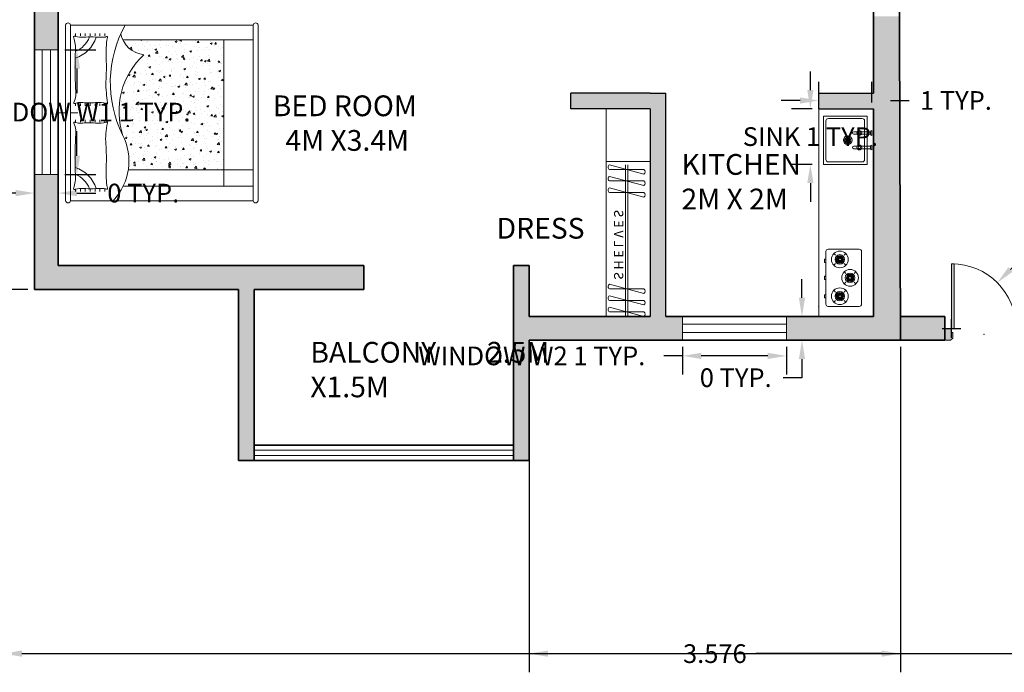
# Model space of a CAD drawing. Units: metres. Extents: x 2031 to 2061.8, y 1886.4 to 1909.8.
# Tile 2 of 10: x 2036.4 to 2045.9, y 1886.4 to 1892.7. Entities that reach past the tile are written whole.
import ezdxf

# ---------------------------------------------------------------- set-up
doc = ezdxf.new("R2010")
doc.units = ezdxf.units.M
for name, color, linetype, lineweight in [('A-ANNO-DIMS', 2, 'Continuous', 18), ('A-AREA-IDEN', 7, 'Continuous', 18), ('A-EQPM', 8, 'Continuous', 18), ('A-FLOR-CASE', 8, 'Continuous', 18), ('A-FLOR-FIXT', 8, 'Continuous', 18), ('A-WALL-PATT', 252, 'Continuous', 13), ('doors & windows', 30, 'Continuous', 18), ('furniture', 24, 'Continuous', 13), ('grills', 5, 'Continuous', 13), ('inner walls', 4, 'Continuous', 25), ('windows', 30, 'Continuous', 18)]:
    doc.layers.add(name, color=color, linetype=linetype, lineweight=lineweight)
doc.layers.add('outer walls', color=1, linetype='Continuous', lineweight=35, plot=False)
doc.styles.get("Standard").update_dxf_attribs({"font": 'arial.ttf'})
doc.dimstyles.get("Standard").update_dxf_attribs({"dimtxt": 0.18, "dimasz": 0.18, "dimexe": 0.18, "dimexo": 0.0625, "dimgap": 0.09, "dimtad": 0, "dimtih": 1, "dimtoh": 1, "dimdec": 4, "dimzin": 0, "dimdsep": 46, "dimtxsty": 'Standard', "dimcen": 0.09, "dimadec": 0, "dimazin": 0, "dimtfac": 1, "dimtdec": 4, "dimtofl": 0, "dimtmove": 0, "dimatfit": 3, "dimfxl": 1, "dimtolj": 1, "dimtzin": 0, "dimarcsym": 0})

# ---------------------------------------------------------------- blocks, each defined once
blk = doc.blocks.new('sink')
for p, q in [((0, 0), (-22.00000000000001, 0)), ((0, 0), (0, 0)), ((-20.00000000000023, -2.999999999999995), (-2.000000000000178, -3)), ((-19.99999999999959, -22.99999999999988), (-20.00000000000023, -2.999999999999995)), ((-18.00000000000017, -3.999999999999996), (-4.000000000000113, -3.999999999999999)), ((-2.000000000000178, -3), (-1.999999999999543, -22.99999999999988)), ((-18.99999999999966, -20.99999999999994), (-19.00000000000017, -4.999999999999996)), ((-3.000000000000114, -5), (-2.999999999999607, -20.99999999999988)), ((-0.5000000000000026, -9.499999999999813), (-7.500000000000004, -9.499999999999812)), ((-0.5000000000000028, -10.49999999999981), (-7.500000000000004, -10.49999999999981)), ((-0.5000000000000026, -9.499999999999813), (-0.5000000000000028, -10.49999999999981)), ((-2.4e-15, -8.999999999999813), (-2.9e-15, -10.99999999999981)), ((-0.500000000000004, -15.49999999999981), (-7.500000000000005, -15.49999999999981)), ((-0.500000000000004, -15.49999999999981), (-0.5000000000000044, -16.49999999999981)), ((-3.9e-15, -14.99999999999981), (-4.4e-15, -16.99999999999981)), ((-0.5000000000000044, -16.49999999999981), (-7.500000000000005, -16.49999999999981)), ((-19.99999999999959, -22.99999999999988), (-1.999999999999543, -22.99999999999988)), ((-17.99999999999966, -21.99999999999988), (-3.999999999999607, -21.99999999999989))]:
    blk.add_line(p, q)
for centre, radius in [((-10.00000000000014, -12.99999999999968), 1.794435724606955), ((-10.00000000000014, -12.99999999999968), 1.294435724606955), ((-10.00000000000014, -12.23682250650668), 0.25), ((-5.180961460384426, -9.999999999999812), 1), ((-5.180961460384426, -9.999999999999812), 0.5), ((-10.66093109696162, -12.61841125325318), 0.25), ((-10.66093109696162, -13.38158874674618), 0.25), ((-10.00000000000014, -12.99999999999968), 0.25), ((-10.00000000000014, -13.76317749349269), 0.25), ((-9.33906890303867, -12.61841125325318), 0.25), ((-9.33906890303867, -13.38158874674618), 0.25), ((-5.180961460384427, -15.99999999999981), 1), ((-5.180961460384427, -15.99999999999981), 0.5)]:
    blk.add_circle(centre, radius)
for centre, radius, start, end in [((-18.00000000000017, -4.999999999999996), 1, 89.99999999999999, 180), ((-4.000000000000115, -5), 1, 0, 89.99999999999999), ((-7.500000000000004, -9.999999999999812), 0.5, 89.99999999999999, 270), ((0.010449978117122, -9.510449978116938), 0.5105569333604445, 91.17280055555744, 178.8271994444424), ((0.0104499781171218, -10.48955002188269), 0.5105569333604445, 181.1728005555574, 268.8271994444423), ((-7.500000000000005, -15.99999999999981), 0.5, 89.99999999999999, 270), ((0.0104499781171206, -15.51044997811693), 0.5105569333604445, 91.17280055555744, 178.8271994444424), ((0.0104499781171203, -16.48955002188269), 0.5105569333604445, 181.1728005555573, 268.8271994444423), ((-17.99999999999966, -20.99999999999988), 1, 180, 270), ((-3.999999999999607, -20.99999999999988), 1, 270, 0)]:
    blk.add_arc(centre, radius, start, end)
blk = doc.blocks.new('stove')
at = {"layer": 'furniture'}
h = blk.add_hatch(dxfattribs=at)
h.set_pattern_fill('HEX', color=256, angle=180, style=0)
h.set_pattern_definition([(360, (23.99999999999982, 24.99999999999816), (1e-16, 0.216506351), [0.125, -0.25]), (119.9999999999999, (23.99999999999982, 24.99999999999816), (-0.1875000000466704, -0.1082531754999999), [0.1249999999999998, -0.2499999999999996]), (59.99999999999994, (24.12499999999982, 24.99999999999816), (-0.1875000000466704, 0.1082531755000001), [0.125, -0.25])])
h.paths.add_polyline_path([(10.36428182591571, 19.71316705046143, 1), (7.364281825915714, 19.71316705046143, 1)])
h.paths.add_polyline_path([(9.364281825915715, 19.71316705046143, -1), (8.364281825915715, 19.71316705046143, -1)], flags=16)
h = blk.add_hatch(dxfattribs=at)
h.set_pattern_fill('HEX', color=256, angle=180, style=0)
h.set_pattern_definition([(180, (-2.000000000000001, 6.713167050462818), (-1e-16, -0.216506351), [0.125, -0.25]), (300, (-2.000000000000001, 6.713167050462818), (0.1875000000466704, 0.1082531754999999), [0.1249999999999999, -0.2499999999999998]), (239.9999999999999, (-2.125000000000001, 6.713167050462818), (0.1875000000466704, -0.1082531755000001), [0.125, -0.25])])
h.paths.add_polyline_path([(14.6357181740841, 11.99999999999954, 1), (11.6357181740841, 11.99999999999954, 1)])
h.paths.add_polyline_path([(12.6357181740841, 11.99999999999954, -1), (13.6357181740841, 11.99999999999954, -1)], flags=16)
h = blk.add_hatch(dxfattribs=at)
h.set_pattern_fill('HEX', color=256, angle=180, style=0)
h.set_pattern_definition([(360, (23.99999999999982, -0.9999999999999342), (-1e-16, -0.216506351), [0.125, -0.25]), (239.9999999999999, (23.99999999999982, -0.9999999999999342), (-0.1875000000466704, 0.1082531755), [0.1249999999999999, -0.2499999999999998]), (300, (24.12499999999982, -0.9999999999999342), (-0.1875000000466704, -0.1082531755), [0.125, -0.2499999999999999])])
h.paths.add_polyline_path([(10.36428182591571, 4.2868329495368, 1), (7.364281825915714, 4.2868329495368, 1)])
h.paths.add_polyline_path([(9.364281825915715, 4.2868329495368, -1), (8.364281825915715, 4.2868329495368, -1)], flags=16)
for p, q in [((3, 1.000000000000003), (3.000000000000007, 22.99999999999909)), ((4.000000000000007, 23.99999999999909), (17, 23.99999999999908)), ((6.389408091762671, 22.18804078461422), (7.09651487294905, 21.48093400342751)), ((10.6320487788818, 21.48093400342809), (11.33915556006851, 22.18804078461447)), ((18, 22.99999999999908), (18, 0.9999999999991327)), ((3.000000000000007, 19.86017834974973), (2.500000000000003, 19.86017834974973)), ((2.500000000000003, 19.86017834974973), (2.500000000000003, 18.36017834974973)), ((2.500000000000003, 18.36017834974973), (3.000000000000003, 18.36017834974973)), ((6.389408091762675, 17.23829331630864), (7.096514872949061, 17.94540009749535)), ((10.63204877888179, 17.94540009749477), (11.3391555600685, 17.23829331630838)), ((2.500000000000003, 12.64999999999954), (2.500000000000003, 11.34999999999955)), ((3.000000000000003, 12.64999999999954), (2.500000000000003, 12.64999999999954)), ((11.36795122111803, 13.7677669529662), (10.66084443993131, 14.47487373415259)), ((15.61059190823715, 14.47487373415233), (14.90348512705075, 13.76776695296562)), ((2.500000000000003, 11.34999999999955), (3.000000000000003, 11.34999999999955)), ((11.36795122111803, 10.23223304703288), (10.66084443993131, 9.525126265846504)), ((15.61059190823714, 9.525126265846753), (14.90348512705077, 10.23223304703346)), ((2.500000000000003, 4.936832949536799), (2.500000000000003, 3.636832949536802)), ((3.000000000000003, 4.936832949536799), (2.500000000000003, 4.936832949536799)), ((6.389408091762671, 6.761706683689592), (7.096514872949061, 6.054599902502877)), ((10.63204877888178, 6.05459990250346), (11.3391555600685, 6.761706683689842)), ((2.500000000000003, 3.636832949536802), (3.000000000000003, 3.636832949536802)), ((16.99999999999994, -8.669e-13), (3.999999999999946, 3.6e-15)), ((6.389408091762668, 1.811959215384014), (7.096514872949043, 2.519065996570723)), ((10.63204877888179, 2.519065996570138), (11.3391555600685, 1.81195921538376))]:
    blk.add_line(p, q, dxfattribs=at)
for centre, radius in [((8.864281825915715, 19.71316705046143), 3.499999999999999), ((8.864281825915715, 19.71316705046143), 1.999999999999999), ((8.864281825915715, 19.71316705046143), 1.5), ((8.864281825915715, 19.71316705046143), 0.5000000000000004), ((13.1357181740841, 11.99999999999954), 3.499999999999999), ((13.1357181740841, 11.99999999999954), 1.999999999999999), ((13.1357181740841, 11.99999999999954), 1.5), ((13.1357181740841, 11.99999999999954), 0.5000000000000004), ((8.864281825915715, 4.286832949536801), 3.499999999999999), ((8.864281825915715, 4.2868329495368), 1.999999999999999), ((8.864281825915715, 4.2868329495368), 1.5), ((8.864281825915715, 4.2868329495368), 0.5000000000000004)]:
    blk.add_circle(centre, radius, dxfattribs=at)
for centre, start, end in [((4.000000000000007, 22.99999999999909), 90, 180), ((17, 22.99999999999908), 0, 90), ((4, 1.000000000000003), 180, 269.9999999999968), ((17, 0.9999999999991331), 269.9999999999968, 0)]:
    blk.add_arc(centre, 1, start, end, dxfattribs=at)
at = {"layer": 'furniture', "ltscale": 9}
blk.add_point((0, 0), dxfattribs=at)
blk = doc.blocks.new('bed')
at = {"layer": 'furniture'}
h = blk.add_hatch(dxfattribs=at)
h.set_pattern_fill('AR-CONC', color=256, angle=-90.00000000000003, style=0)
h.set_pattern_definition([(320, (0, 2.380000000001032), (-0.6275213498259539, -7.172601826007534), [0.75, -8.25]), (265, (0, 2.380000000001032), (7.521921337000119, 1.387513336129997), [0.6, -6.599999999999999]), (10.45139999999999, (-0.0522933999999964, 1.782283200001032), (6.894395420609534, -5.785093817140218), [0.6374019000000001, -7.011421119999999]), (316.1842, (2, 2.380000000001032), (-1.655190143290184, -10.67241048625644), [1.125, -12.375]), (6.635599999999979, (1.862066929999997, 1.490632550001038), (9.741178709004412, -9.346627055487035), [0.956102879999999, -10.51712999999998]), (261.1842, (2, 2.380000000001032), (9.741186009253243, -9.346619451336275), [0.8999999999999989, -9.899999999999984]), (291, (1.5, 1.380000000001032), (-4.02618890665339, -5.969070521184614), [0.75, -8.25]), (236, (1.5, 1.380000000001032), (7.251500450468529, -2.433153319215819), [0.6, -6.599999999999999]), (341.4514, (1.164483939999996, 0.8825776700010266), (3.22530496709952, -8.402226285814901), [0.6374019000000001, -7.011421119999999]), (307.4999999999999, (0, 2.380000000001032), (3.328938538313114, -0.121598553172908), [0, -6.519999999999999, 0, -6.7, 0, -6.625]), (277.5, (0, 2.380000000001032), (3.944117118823601, -2.630695374421487), [0, -3.819999999999999, 0, -6.37, 0, -2.524999999999999]), (237.5, (0, 4.610000000001036), (-0.2255487173438, -5.33822436172409), [0, -2.5, 0, -7.799999999999999, 0, -10.35]), (227.5, (0, 5.610000000001036), (1.001049823323174, -5.831861693423862), [0, -3.25, 0, -5.179999999999999, 0, -7.349999999999999])])
h.paths.add_polyline_path([(30.01221964123038, -67.99999999999999), (30.01221964123036, -26.4972098666525, 0.2630430180581192), (23.90476957024844, -35.1500155485824, 0.2934236934375176), (-9.177957282599145, -26.46678060096597, -0.1566832162072435), (-23.39221964123496, -28.71851562074189), (-23.39221964123494, -67.99999999999999)])
for p, q in [((0, -3), (0, 0)), ((36.01221964123033, -3), (-36.01221964123033, -3)), ((-36.01221964123033, -5.000000000000028), (-36.01221964123027, -80)), ((36.01221964123033, -5.000000000000042), (-36.01221964123033, -5.000000000000028)), ((-31.23716250644156, -7.067621994530554), (-32.23716250644157, -7.067621994530554)), ((-3.810600647213163, -7.067621994530554), (-2.810600647213163, -7.067621994530554)), ((0, -8.000000000000043), (0, -5.000000000000042)), ((3.894900133777696, -7.067621994530526), (2.894900133777696, -7.067621994530526)), ((31.62837541028949, -7.067621994530526), (32.62837541028949, -7.067621994530526)), ((36.01221964123039, -79.99999999999999), (36.01221964123033, -5.000000000000042)), ((-31.23716250644156, -9.067621994530555), (-32.23716250644157, -9.067621994530555)), ((-31.23716250644156, -11.06762199453055), (-32.23716250644157, -11.06762199453055)), ((-3.810600647213163, -9.067621994530555), (-2.810600647213163, -9.067621994530555)), ((-3.810600647213163, -11.06762199453055), (-2.810600647213163, -11.06762199453055)), ((3.894900133777696, -9.067621994530526), (2.894900133777696, -9.067621994530526)), ((3.894900133777696, -11.06762199453052), (2.894900133777696, -11.06762199453052)), ((31.62837541028949, -9.067621994530526), (32.62837541028949, -9.067621994530526)), ((31.62837541028949, -11.06762199453052), (32.62837541028949, -11.06762199453052)), ((-31.23716250644156, -13.06762199453055), (-32.23716250644157, -13.06762199453055)), ((-31.23716250644156, -15.06762199453055), (-32.23716250644157, -15.06762199453055)), ((-3.810600647213163, -13.06762199453055), (-2.810600647213163, -13.06762199453055)), ((-3.810600647213163, -15.06762199453055), (-2.810600647213163, -15.06762199453055)), ((3.894900133777696, -13.06762199453052), (2.894900133777696, -13.06762199453052)), ((3.894900133777696, -15.06762199453052), (2.894900133777696, -15.06762199453052)), ((31.62837541028949, -13.06762199453052), (32.62837541028949, -13.06762199453052)), ((31.62837541028949, -15.06762199453052), (32.62837541028949, -15.06762199453052)), ((-31.23716250644156, -17.06762199453055), (-32.23716250644157, -17.06762199453055)), ((-31.23716250644156, -19.06762199453055), (-32.23716250644157, -19.06762199453055)), ((-3.810600647213163, -17.06762199453055), (-2.810600647213163, -17.06762199453055)), ((-3.810600647213163, -19.06762199453055), (-2.810600647213163, -19.06762199453055)), ((3.894900133777696, -17.06762199453052), (2.894900133777696, -17.06762199453052)), ((3.894900133777696, -19.06762199453052), (2.894900133777696, -19.06762199453052)), ((31.62837541028949, -17.06762199453052), (32.62837541028949, -17.06762199453052)), ((31.62837541028949, -19.06762199453052), (32.62837541028949, -19.06762199453052)), ((-36.01221964123027, -80), (36.01221964123039, -79.99999999999997)), ((-36.01221964123027, -82), (36.01221964123039, -82))]:
    blk.add_line(p, q, dxfattribs=at)
at = {"layer": 'furniture', "ltscale": 5}
blk.add_line((-30.0122196412303, -26.65900214866815), (-30.01221964123028, -80), dxfattribs=at)
at = {"layer": 'furniture', "ltscale": 7}
blk.add_line((30.01221964123039, -79.99999999999999), (30.01221964123036, -26.4972098666525), dxfattribs=at)
at = {"layer": 'furniture', "ltscale": 0.3}
for p, q in [((-23.39221964123493, -80.00000000000003), (-23.39221964123496, -28.71851562074188)), ((-30.01221964123028, -67.99999999999999), (30.01221964123039, -67.99999999999999))]:
    blk.add_line(p, q, dxfattribs=at)
at = {"layer": 'furniture'}
for centre, radius, start, end in [((-35.95310404783035, -4.000000000000014), 1.001745802777857, 93.38313670775338, 266.6168632922466), ((35.95310404783047, -4.000000000000014), 1.001745802777857, 273.3831367077534, 86.61686329224663), ((-31.09685452420217, -6.56812628935117), 0.3815901177143176, 35.89755946985184, 208.6271807330242), ((-44.4434251214767, -13.85312857714783), 14.82374463825802, 27.16285943351717, 28.62718073212637), ((-46.75951437957865, -9.65138206848897), 15.71579241958107, 357.4803608088326, 9.395608387614068), ((-34.45294545533051, -3.506108501804959), 9.853247350176973, 289.8695209624031, 338.9842964810487), ((-34.45294545533051, -3.506108501804959), 12.47479548168961, 286.0319050224358, 344.1205283884622), ((-26.34909713879518, 6.677823774407073), 13.75788850886336, 251.1782289026713, 273.3982224065857), ((-18.01528168092849, -163.5963416214672), 156.7209082093599, 87.00321809951629, 92.74968346925495), ((-8.031939823939297, 2.030581047412752), 9.294330538692307, 258.8960367609226, 294.7184225587751), ((0.254091396095987, -8.800915214962217), 4.494229367051207, 159.014640107615, 186.2730421081171), ((-4.029449448298862, -6.668977911985379), 0.2818061021667602, 335.7259061638442, 114.3030308467571), ((3.223958981487498, -9.94006998173215), 7.675076275868892, 155.7259061638442, 159.0146401085631), ((4.113748934860268, -6.668977911985379), 0.2818061021635516, 65.69696915417202, 204.2740938370052), ((-3.139659494904833, -9.940069981732137), 7.675076275868892, 20.98535989143595, 24.27409383615427), ((-0.1697919095242355, -8.800915214962217), 4.494229367051207, 353.7269578918828, 20.98535989238499), ((8.116239310533615, 2.030581047735168), 9.294330539002221, 245.2815774418415, 281.1039632384965), ((18.09958116748922, -163.5963416214399), 156.7209082093326, 87.2503165307418, 92.99678190048373), ((34.53724494190226, -3.506108501789682), 12.47479548168961, 195.8794716115377, 253.9680949775642), ((34.53724494190226, -3.506108501789682), 9.853247350176973, 201.0157035189505, 250.1304790375968), ((26.43339662535652, 6.677823774423444), 13.75788850886336, 266.6017775934111, 288.8217710973251), ((31.18115401076358, -6.568126289351184), 0.3815901177179044, 331.3728192669758, 144.1024405301472), ((46.84381386614001, -9.651382068520647), 15.71579241958353, 170.6043916115409, 182.5196391911672), ((44.52772460803806, -13.85312857714784), 14.82374463825802, 151.3728192678729, 152.8371405664821), ((-28.61556435462791, 31.03444768063454), 42.31456350822244, 266.4835611990511, 266.6487421238194), ((54.88285648445511, -13.16191061182081), 85.98801403775587, 178.1208768196816, 183.3613129440673), ((-32.81622258778788, -12.43616332427339), 28.77528664700029, 354.3784002715227, 6.27304210895588), ((32.90052207435963, -12.43616332427341), 28.77528664700055, 173.7269578910441, 185.6215997284773), ((-54.79855699787332, -13.1619106118885), 85.98801403775471, 356.6386870559327, 1.87912318031836), ((28.69986384117891, 31.03444768073385), 42.31456350831875, 273.3512578762066, 273.5164388009489), ((12.27920019974715, -16.10835590841725), 16.48064095036883, 177.0317121189266, 192.8677860199701), ((-12.19490071317551, -16.10835590841725), 16.48064095036894, 347.1322139800299, 2.968287881073314), ((-31.05019458355673, -19.91479358257859), 0.2912925215689113, 147.6219291273817, 311.93432899363), ((-33.19532486499685, -18.55460390606353), 2.248727139855352, 327.6219291288709, 339.224552802207), ((-34.12771521855714, -18.41167218428833), 3.177308659740759, 342.7808628527732, 3.755021134780372), ((-24.39731400277299, -58.0065508966982), 38.42172354635978, 93.51643880178425, 99.67664784205135), ((-24.51665474671893, -56.06449133928439), 36.47600066328987, 86.48356119821578, 93.51643880178425), ((-18.48842024981553, 70.49496359167773), 90.23180174042126, 267.5920770069633, 273.6328801943956), ((-10.30534078399284, -44.95285539311296), 25.51674577343078, 75.95197577712642, 95.54518109318596), ((-3.947726608991956, -19.99033763805275), 0.2654728058058112, 231.9004795059564, 52.89022406852256), ((4.032026095563765, -19.99033763805275), 0.2654728058058112, 127.1097759314774, 308.0995204940429), ((7.570216687580227, -34.67789736270967), 14.86666553287629, 87.39755039330738, 103.1191401867811), ((11.43897390287765, -34.80624327566366), 15.31635237680183, 84.69404282866213, 102.035481886755), ((18.57271973638731, 70.4949635916777), 90.23180174042125, 266.3671198056044, 272.4079229930367), ((24.6009542333012, -56.0644913392844), 36.47600066328987, 86.48356119821578, 93.51643880178425), ((24.48161348934542, -58.00655089669821), 38.42172354635978, 80.32335215794863, 86.48356119821578), ((31.13449407013883, -19.91479358255678), 0.2912925215689113, 228.06567100637, 32.37807087261824), ((34.21201470513921, -18.41167218428845), 3.177308659740705, 176.2449788652196, 197.2191371472267), ((33.27962435157895, -18.55460390604825), 2.248727139855352, 200.775447197793, 212.378070871129), ((-19.78970084288576, -5.469494448941333), 23.52647715105876, 226.4060518471351, 297.4441169484015), ((12.50744191168894, -69.71437404891591), 48.3828132966499, 60.93454900685955, 116.3226601669859), ((0.602167516954296, -56.56840710701565), 31.65057281321388, 42.58740832788977, 108.5033645785765), ((34.6132349005153, -36.22659364526982), 10.76244628919441, 101.1719081394, 174.2590453022261), ((-35.95310404783035, -81), 1.001745802777857, 93.38313670775338, 266.6168632922466), ((35.95310404783044, -81), 1.001745802777857, 273.3831367077534, 86.61686329224663)]:
    blk.add_arc(centre, radius, start, end, dxfattribs=at)
blk = doc.blocks.new('hangers')
at = {"layer": 'furniture'}
for p, q in [((1.8e-15, 16.5), (4.000000000000001, 1.5)), ((2.000000000000001, 16.5), (2.000000000000001, 1.5)), ((5.000000000000001, 16.5), (9.000000000000002, 1.5)), ((7.000000000000001, 16.5), (7.000000000000001, 1.5)), ((10, 16.5), (14, 1.5)), ((12, 16.5), (12, 1.5)), ((52, 16.5), (56, 1.5)), ((54, 16.5), (54, 1.5)), ((57, 16.5), (61, 1.5)), ((59, 16.5), (59, 1.5)), ((62, 16.5), (66, 1.5)), ((64, 16.5), (64, 1.5)), ((66, 9.5), (1.8e-15, 9.5)), ((1.8e-15, 8.5), (66, 8.5))]:
    blk.add_line(p, q, dxfattribs=at)
for centre, radius, start, end in [((1.000000000000001, 15.6218374153911), 1.33085293139661, 41.28839256573093, 138.711607434269), ((6.000000000000001, 15.6218374153911), 1.33085293139661, 41.28839256573093, 138.711607434269), ((11, 15.6218374153911), 1.33085293139661, 41.28839256573093, 138.711607434269), ((53, 15.6218374153911), 1.33085293139661, 41.28839256573107, 138.7116074342689), ((58, 15.6218374153911), 1.33085293139661, 41.28839256573107, 138.7116074342689), ((63, 15.6218374153911), 1.33085293139661, 41.28839256573107, 138.7116074342689), ((3.000000000000001, 1.915335972440686), 1.082822224561017, 202.5548696812492, 337.4451303187508), ((8.000000000000002, 1.915335972440686), 1.082822224561017, 202.5548696812492, 337.4451303187508), ((13, 1.915335972440686), 1.082822224561017, 202.5548696812492, 337.4451303187508), ((55, 1.915335972440686), 1.082822224561017, 202.5548696812491, 337.4451303187509), ((60, 1.915335972440686), 1.082822224561017, 202.5548696812491, 337.4451303187509), ((65, 1.915335972440686), 1.082822224561017, 202.5548696812491, 337.4451303187509)]:
    blk.add_arc(centre, radius, start, end, dxfattribs=at)
blk.add_point((0, 0), dxfattribs=at)
blk.add_text('S H E L V E S', height=4, dxfattribs=at).set_placement((15.9969173169515, 3.475366291579639))
blk = doc.blocks.new('D2')
at = {"layer": 'doors & windows'}
h = blk.add_hatch(dxfattribs=at)
h.set_pattern_fill('DOTS', color=256, scale=2, angle=180, style=0)
h.set_pattern_definition([(180, (0, -3.999999999998181), (-0.0625, -0.125), [0, -0.125])])
h.paths.add_polyline_path([(2.5, 1.819e-12), (3.5, 1.819e-12), (3.500000000001818, 24.97999199359535, 0.0100030022021123), (2.500000000001818, 25.00000000000182)])
h = blk.add_hatch(dxfattribs=at)
h.set_pattern_fill('DOTS', color=256, scale=2, angle=180, style=0)
h.set_pattern_definition([(180, (0, 0), (-0.0625, -0.125), [0, -0.125])])
edge = h.paths.add_edge_path()
edge.add_line((27.50000000000182, 1.819e-12), (27.50000000000182, -1.499999999998181))
edge.add_line((27.50000000000182, -1.499999999998181), (27.00000000000157, -1.499999999998181))
edge.add_line((27.00000000000157, -1.499999999998181), (27.00000000000039, -3.749999999998181))
edge.add_line((27.00000000000039, -3.749999999998181), (27.25, -3.749999999998181))
edge.add_arc((27.75893604593965, -3.741063954058532), 0.5090144907305875, 181.0059124648427, 268.9940875351573)
edge.add_line((27.75, -4.249999999998181), (27.75, -4.499999999998181))
edge.add_line((27.75, -4.499999999998181), (30.00000000000182, -4.499999999998181))
edge.add_line((30.00000000000182, -4.499999999998181), (30.00000000000182, 0))
edge.add_line((30.00000000000182, 0), (27.50000000000182, 1.819e-12))
edge = h.paths.add_edge_path()
edge.add_line((2.5, -1.499999999998181), (2.5, 1.819e-12))
edge.add_line((2.5, 1.819e-12), (1.819e-12, 0))
edge.add_line((1.819e-12, 0), (0, -4.499999999998181))
edge.add_line((0, -4.499999999998181), (2.250000000001548, -4.499999999998181))
edge.add_line((2.250000000001548, -4.499999999998181), (2.250000000001548, -4.249999999998181))
edge.add_arc((2.2410639540619, -3.741063954058532), 0.5090144907305875, 271.0059124648427, 358.9940875351573)
edge.add_line((2.750000000001548, -3.749999999998181), (3, -3.749999999998181))
edge.add_line((3, -3.749999999998181), (3, -1.499999999998181))
edge.add_line((3, -1.499999999998181), (2.5, -1.499999999998181))
for p, q in [((1.819e-12, 0), (0, -4.499999999998181)), ((30.00000000000182, 0), (30.00000000000182, -4.499999999998181))]:
    blk.add_line(p, q)
blk.add_lwpolyline([(3.5, 1.819e-12), (3.500000000001818, 25.00000000000182), (2.500000000001818, 25.00000000000182), (2.5, 1.819e-12)], close=True, dxfattribs=at)
for points in [[(3, -3.749999999998181), (3, -1.499999999998181), (2.5, -1.499999999998181), (2.5, 1.819e-12), (1.819e-12, 0)], [(27.00000000000039, -3.749999999998181), (27.00000000000182, -1.499999999998181), (27.50000000000182, -1.499999999998181), (27.50000000000182, 1.819e-12), (30, 0)], [(0, -4.499999999998181), (2.250000000001548, -4.499999999998181)], [(30, -4.499999999998181), (27.75, -4.499999999998181)]]:
    blk.add_lwpolyline(points, dxfattribs=at)
for points in [[(2.250000000001548, -4.499999999998181), (2.250000000001548, -4.249999999998181, 0.4039662087126686), (2.750000000001548, -3.749999999998181), (3.000000000001548, -3.749999999998181)], [(27.75, -4.499999999998181), (27.75, -4.249999999998181, -0.4039662087126686), (27.25, -3.749999999998181), (27, -3.749999999998181)]]:
    blk.add_lwpolyline(points, format="xyb", dxfattribs=at)
at = {"layer": 'doors & windows', "ltscale": 6}
blk.add_arc((2.5, 1.819e-12), 25, 0, 90, dxfattribs=at)
at = {"layer": 'doors & windows'}
blk.add_point((15, -2.24999999999909), dxfattribs=at)
blk = doc.blocks.new('WIN-1200')
for p, q in [((0.2299999999995634, 1.200000000000045), (-4.547e-13, 1.199999999999818)), ((0.0750000000007276, -2.274e-13), (0.0749999999995907, 1.200000000000045)), ((0.1550000000006548, -2.274e-13), (0.154999999999518, 1.200000000000045)), ((0.2300000000007003, 0), (6.821e-13, -2.274e-13))]:
    blk.add_line(p, q)
blk = doc.blocks.new('WIN-1000')
for p, q in [((2.274e-13, 0), (0, 0.2299999999997908)), ((1.000000000000227, 9.095e-13), (1, 0.2300000000007003)), ((2.274e-13, 0.1549999999997453), (1.000000000000227, 0.1549999999997453)), ((2.274e-13, 0.0749999999998181), (1.000000000000227, 0.0749999999998181))]:
    blk.add_line(p, q)
blk = doc.blocks.new('BALCONY-GUARD-2500')
for p, q in [((4.547e-13, 0.0500000000010914), (2.5, 0.0500000000006367)), ((4.547e-13, 6.821e-13), (2.5, 4.547e-13))]:
    blk.add_line(p, q)
blk = doc.blocks.new('*D20')
at = {"layer": 'A-ANNO-DIMS', "color": 0, "lineweight": -2, "transparency": 16777216}
for p, q in [((2036.825693535109, 1892.386538828238), (2037.12319353511, 1892.386538828238)), ((2036.94319353511, 1892.206538828238), (2036.94319353511, 1891.96966979686)), ((2036.94319353511, 1891.366538828238), (2036.94319353511, 1891.603407859615)), ((2036.825693535109, 1891.186538828237), (2037.12319353511, 1891.186538828237))]:
    blk.add_line(p, q, dxfattribs=at)
at = {"layer": 'A-ANNO-DIMS', "color": 0, "transparency": 16777216}
for points in [[(2036.91319353511, 1892.206538828238), (2036.97319353511, 1892.206538828238), (2036.94319353511, 1892.386538828238)], [(2036.91319353511, 1891.366538828238), (2036.97319353511, 1891.366538828238), (2036.94319353511, 1891.186538828237)]]:
    blk.add_solid(points, dxfattribs=at)
at = {"layer": 'Defpoints', "color": 0, "transparency": 16777216}
for p in [(2036.763193535109, 1892.386538828238), (2036.94319353511, 1892.386538828238), (2036.763193535109, 1891.186538828237)]:
    blk.add_point(p, dxfattribs=at)
at = {"layer": 'A-ANNO-DIMS', "color": 0, "transparency": 16777216, "insert": (2036.94319353511, 1891.786538828236), "char_height": 0.18, "attachment_point": 5}
blk.add_mtext('\\A1;WINDOW W1 1 TYP.', dxfattribs=at)
blk = doc.blocks.new('*D21')
at = {"layer": 'A-ANNO-DIMS', "color": 0, "lineweight": -2, "transparency": 16777216}
for p, q in [((2036.533193535106, 1891.124038828237), (2036.533193535106, 1890.826538828237)), ((2036.763193535108, 1891.124038828237), (2036.763193535108, 1890.826538828237)), ((2036.353193535106, 1891.006538828237), (2036.173193535107, 1891.006538828237)), ((2036.943193535108, 1891.006538828237), (2037.123193535109, 1891.006538828237))]:
    blk.add_line(p, q, dxfattribs=at)
at = {"layer": 'A-ANNO-DIMS', "color": 0, "transparency": 16777216}
for points in [[(2036.353193535106, 1891.036538828237), (2036.353193535106, 1890.976538828237), (2036.533193535106, 1891.006538828237)], [(2036.943193535108, 1891.036538828237), (2036.943193535108, 1890.976538828237), (2036.763193535108, 1891.006538828237)]]:
    blk.add_solid(points, dxfattribs=at)
at = {"layer": 'Defpoints', "color": 0, "transparency": 16777216}
for p in [(2036.533193535106, 1891.186538828237), (2036.763193535108, 1891.186538828237), (2036.763193535108, 1891.006538828237)]:
    blk.add_point(p, dxfattribs=at)
at = {"layer": 'A-ANNO-DIMS', "color": 0, "transparency": 16777216, "insert": (2037.581358610142, 1891.006538828237), "char_height": 0.18, "attachment_point": 5}
blk.add_mtext('\\A1;0 TYP.', dxfattribs=at)
blk = doc.blocks.new('*D24')
at = {"layer": 'A-ANNO-DIMS', "color": 0, "lineweight": -2, "transparency": 16777216}
for p, q in [((2044.00555249375, 1891.998154600067), (2044.00555249375, 1892.178154600067)), ((2044.023319853971, 1891.818154600067), (2043.82555249375, 1891.818154600067)), ((2044.023319853971, 1891.283038865253), (2043.82555249375, 1891.283038865253)), ((2044.00555249375, 1891.103038865253), (2044.00555249375, 1890.923038865253))]:
    blk.add_line(p, q, dxfattribs=at)
at = {"layer": 'A-ANNO-DIMS', "color": 0, "transparency": 16777216}
for points in [[(2043.975552493749, 1891.998154600067), (2044.035552493749, 1891.998154600067), (2044.00555249375, 1891.818154600067)], [(2043.975552493749, 1891.103038865253), (2044.035552493749, 1891.103038865253), (2044.00555249375, 1891.283038865253)]]:
    blk.add_solid(points, dxfattribs=at)
at = {"layer": 'Defpoints', "color": 0, "transparency": 16777216}
for p in [(2044.00555249375, 1891.818154600067), (2044.08581985397, 1891.818154600067), (2044.08581985397, 1891.283038865253)]:
    blk.add_point(p, dxfattribs=at)
at = {"layer": 'A-ANNO-DIMS', "color": 0, "transparency": 16777216, "insert": (2044.00555249375, 1891.550596732659), "char_height": 0.18, "attachment_point": 5}
blk.add_mtext('\\A1;SINK 1 TYP.', dxfattribs=at)
blk = doc.blocks.new('*D25')
at = {"layer": 'A-ANNO-DIMS', "color": 0, "lineweight": -2, "transparency": 16777216}
for p, q in [((2044.08581985397, 1891.880654600066), (2044.08581985397, 1892.078421960288)), ((2044.59766968727, 1891.880654600066), (2044.59766968727, 1892.078421960288)), ((2043.90581985397, 1891.898421960288), (2043.725819853969, 1891.898421960288)), ((2044.77766968727, 1891.898421960288), (2044.95766968727, 1891.898421960288))]:
    blk.add_line(p, q, dxfattribs=at)
at = {"layer": 'A-ANNO-DIMS', "color": 0, "transparency": 16777216}
for points in [[(2043.90581985397, 1891.928421960288), (2043.90581985397, 1891.868421960288), (2044.08581985397, 1891.898421960288)], [(2044.77766968727, 1891.928421960288), (2044.77766968727, 1891.868421960288), (2044.59766968727, 1891.898421960288)]]:
    blk.add_solid(points, dxfattribs=at)
at = {"layer": 'Defpoints', "color": 0, "transparency": 16777216}
for p in [(2044.08581985397, 1891.818154600066), (2044.59766968727, 1891.898421960288), (2044.59766968727, 1891.818154600066)]:
    blk.add_point(p, dxfattribs=at)
at = {"layer": 'A-ANNO-DIMS', "color": 0, "transparency": 16777216, "insert": (2045.407362729562, 1891.898421960288), "char_height": 0.18, "attachment_point": 5}
blk.add_mtext('\\A1;1 TYP.', dxfattribs=at)
blk = doc.blocks.new('*D40')
at = {"layer": 'A-ANNO-DIMS', "color": 0, "lineweight": -2, "transparency": 16777216}
for p, q in [((2042.774930947017, 1889.438154600063), (2042.594930947017, 1889.438154600063)), ((2042.774930947017, 1889.525654600063), (2042.774930947017, 1889.258154600063)), ((2043.594930947017, 1889.438154600063), (2042.954930947017, 1889.438154600063)), ((2043.774930947017, 1889.525654600063), (2043.774930947017, 1889.258154600063))]:
    blk.add_line(p, q, dxfattribs=at)
at = {"layer": 'A-ANNO-DIMS', "color": 0, "transparency": 16777216}
for points in [[(2042.954930947017, 1889.468154600063), (2042.954930947017, 1889.408154600063), (2042.774930947017, 1889.438154600063)], [(2043.594930947017, 1889.468154600063), (2043.594930947017, 1889.408154600063), (2043.774930947017, 1889.438154600063)]]:
    blk.add_solid(points, dxfattribs=at)
at = {"layer": 'Defpoints', "color": 0, "transparency": 16777216}
for p in [(2042.774930947017, 1889.588154600063), (2043.774930947017, 1889.588154600063), (2042.774930947017, 1889.438154600063)]:
    blk.add_point(p, dxfattribs=at)
at = {"layer": 'A-ANNO-DIMS', "color": 0, "transparency": 16777216, "insert": (2041.322959596403, 1889.438154600063), "char_height": 0.18, "attachment_point": 5}
blk.add_mtext('\\A1;WINDOW W2 1 TYP.', dxfattribs=at)
blk = doc.blocks.new('*D41')
at = {"layer": 'A-ANNO-DIMS', "color": 0, "lineweight": -2, "transparency": 16777216}
for p, q in [((2043.924930947019, 1889.998154600065), (2043.924930947019, 1890.178154600065)), ((2043.837430947018, 1889.818154600065), (2044.104930947019, 1889.818154600065)), ((2043.837430947018, 1889.588154600064), (2044.104930947019, 1889.588154600064)), ((2043.924930947019, 1889.408154600064), (2043.924930947019, 1889.228154600064)), ((2043.924930947019, 1889.228154600064), (2043.744930947019, 1889.228154600064))]:
    blk.add_line(p, q, dxfattribs=at)
at = {"layer": 'A-ANNO-DIMS', "color": 0, "transparency": 16777216}
for points in [[(2043.894930947019, 1889.998154600065), (2043.954930947019, 1889.998154600065), (2043.924930947019, 1889.818154600065)], [(2043.894930947019, 1889.408154600064), (2043.954930947019, 1889.408154600064), (2043.924930947019, 1889.588154600064)]]:
    blk.add_solid(points, dxfattribs=at)
at = {"layer": 'Defpoints', "color": 0, "transparency": 16777216}
for p in [(2043.774930947018, 1889.818154600065), (2043.774930947018, 1889.588154600064), (2043.924930947019, 1889.588154600064)]:
    blk.add_point(p, dxfattribs=at)
at = {"layer": 'A-ANNO-DIMS', "color": 0, "transparency": 16777216, "insert": (2043.286765871985, 1889.228154600063), "char_height": 0.18, "attachment_point": 5}
blk.add_mtext('\\A1;0 TYP.', dxfattribs=at)
blk = doc.blocks.new('*D44')
at = {"layer": 'A-ANNO-DIMS', "color": 0, "lineweight": -2, "transparency": 16777216}
for p, q in [((2036.232783, 1900.719895), (2036.232783, 1886.390195)), ((2056.453886, 1889.9931), (2056.453886, 1886.390195)), ((2036.412783, 1886.570195), (2045.94901662824, 1886.570195)), ((2056.273886, 1886.570195), (2046.73765237176, 1886.570195))]:
    blk.add_line(p, q, dxfattribs=at)
at = {"layer": 'A-ANNO-DIMS', "color": 0, "transparency": 16777216}
for points in [[(2036.412783, 1886.600195), (2036.412783, 1886.540195), (2036.232783, 1886.570195)], [(2056.273886, 1886.600195), (2056.273886, 1886.540195), (2056.453886, 1886.570195)]]:
    blk.add_solid(points, dxfattribs=at)
at = {"layer": 'Defpoints', "color": 0, "transparency": 16777216}
for p in [(2036.232783, 1900.782395), (2056.453886, 1890.0556), (2056.453886, 1886.570195)]:
    blk.add_point(p, dxfattribs=at)
at = {"layer": 'A-ANNO-DIMS', "color": 0, "transparency": 16777216, "insert": (2046.3433345, 1886.570195), "char_height": 0.18, "attachment_point": 5}
blk.add_mtext('\\A1;20.22', dxfattribs=at)
blk = doc.blocks.new('*D54')
at = {"layer": 'A-ANNO-DIMS', "color": 0, "lineweight": -2, "transparency": 16777216}
for p, q in [((2036.670694000001, 1895.341213000001), (2031.564780000002, 1895.341213000001)), ((2031.744780000002, 1895.161213000001), (2031.744780000002, 1892.892034637791)), ((2031.744780000002, 1890.259050000001), (2031.744780000002, 1892.528228362211)), ((2036.470694000001, 1890.079050000001), (2031.564780000002, 1890.079050000001))]:
    blk.add_line(p, q, dxfattribs=at)
at = {"layer": 'A-ANNO-DIMS', "color": 0, "transparency": 16777216}
for points in [[(2031.714780000002, 1895.161213000001), (2031.774780000002, 1895.161213000001), (2031.744780000002, 1895.341213000001)], [(2031.714780000002, 1890.259050000001), (2031.774780000002, 1890.259050000001), (2031.744780000002, 1890.079050000001)]]:
    blk.add_solid(points, dxfattribs=at)
at = {"layer": 'Defpoints', "color": 0, "transparency": 16777216}
for p in [(2036.733194000001, 1895.341213000001), (2031.744780000002, 1890.079050000001), (2036.533194000001, 1890.079050000001)]:
    blk.add_point(p, dxfattribs=at)
at = {"layer": 'A-ANNO-DIMS', "color": 0, "transparency": 16777216, "insert": (2031.744780000002, 1892.7101315), "char_height": 0.18, "attachment_point": 5}
blk.add_mtext('\\A1;5.262', dxfattribs=at)
blk = doc.blocks.new('*D55')
at = {"layer": 'A-ANNO-DIMS', "color": 0, "lineweight": -2, "transparency": 16777216}
for p, q in [((2041.298194, 1889.525655), (2041.298194, 1886.390195)), ((2044.873859, 1889.525655), (2044.873859, 1886.390195)), ((2041.478194, 1886.570195), (2042.69244532674, 1886.570195)), ((2044.693859, 1886.570195), (2043.479607673261, 1886.570195))]:
    blk.add_line(p, q, dxfattribs=at)
at = {"layer": 'A-ANNO-DIMS', "color": 0, "transparency": 16777216}
for points in [[(2041.478194, 1886.600195), (2041.478194, 1886.540195), (2041.298194, 1886.570195)], [(2044.693859, 1886.600195), (2044.693859, 1886.540195), (2044.873859, 1886.570195)]]:
    blk.add_solid(points, dxfattribs=at)
at = {"layer": 'Defpoints', "color": 0, "transparency": 16777216}
for p in [(2041.298194, 1889.588155), (2044.873859, 1889.588155), (2044.873859, 1886.570195)]:
    blk.add_point(p, dxfattribs=at)
at = {"layer": 'A-ANNO-DIMS', "color": 0, "transparency": 16777216, "insert": (2043.086026500001, 1886.570195), "char_height": 0.18, "attachment_point": 5}
blk.add_mtext('\\A1;3.576', dxfattribs=at)
blk = doc.blocks.new('*D65')
at = {"layer": 'A-ANNO-DIMS', "color": 0, "lineweight": -2, "transparency": 16777216}
for p, q in [((2046.070887774461, 1890.408268174999), (2045.933100891741, 1890.270283483999)), ((2046.250887774462, 1890.408268174999), (2046.070887774461, 1890.408268174999)), ((2045.364289, 1889.610655), (2045.364289000001, 1889.790655)), ((2045.274289, 1889.700655), (2045.454289, 1889.700655))]:
    blk.add_line(p, q, dxfattribs=at)
at = {"layer": 'A-ANNO-DIMS', "color": 0, "transparency": 16777216}
blk.add_solid([(2045.911872477741, 1890.291481465956), (2045.954329305741, 1890.249085502042), (2045.805913, 1890.142913)], dxfattribs=at)
at = {"layer": 'Defpoints', "color": 0, "transparency": 16777216}
for p in [(2045.805913, 1890.142913), (2045.364289, 1889.700655)]:
    blk.add_point(p, dxfattribs=at)
at = {"layer": 'A-ANNO-DIMS', "color": 0, "transparency": 16777216, "insert": (2046.926317515253, 1890.408268174999), "char_height": 0.18, "attachment_point": 5}
blk.add_mtext('\\A1;2X R0.625', dxfattribs=at)

msp = doc.modelspace()

# ---------------------------------------------------------------- hatches: boundary and pattern name
at = {"layer": 'A-WALL-PATT'}
h = msp.add_hatch(color=256, dxfattribs=at)
h.dxf.hatch_style = 1
h.paths.add_polyline_path([(2036.763193535108, 1893.70904977034), (2039.913193535109, 1893.70904977034), (2039.913193535108, 1893.85904977034), (2038.113193535108, 1893.85904977034), (2038.113193535108, 1894.400131167244), (2037.963193535108, 1894.400131167244), (2037.963193535108, 1893.85904977034), (2036.533193535108, 1893.85904977034), (2036.533193535108, 1892.386538828237), (2036.763193535108, 1892.386538828237)])
h.paths.add_polyline_path([(2038.113193535108, 1895.341212564149), (2037.963193535108, 1895.341212564149), (2037.963193535108, 1894.900131167244), (2038.113193535108, 1894.900131167244)])
h.paths.add_polyline_path([(2043.41320216943, 1895.579519242849), (2040.763193535108, 1895.571212564149), (2040.415704939613, 1895.571212564149), (2040.415704939613, 1895.341212564148), (2040.613193535108, 1895.341212564148), (2040.613193535108, 1893.70904977034), (2040.763193535108, 1893.70904977034), (2040.763193535108, 1895.341212564148), (2043.413949162095, 1895.341212564148)])
h.paths.add_polyline_path([(2039.705693535108, 1890.30904977034), (2036.763193535108, 1890.30904977034), (2036.763193535108, 1891.186538828237), (2036.533193535108, 1891.186538828237), (2036.533193535108, 1890.07904977034), (2038.498193535108, 1890.07904977034), (2038.498193535108, 1888.42904977034), (2038.648193535108, 1888.42904977034), (2038.648193535108, 1890.07904977034), (2039.705693535108, 1890.07904977034)])
h.paths.add_polyline_path([(2042.774930947016, 1889.818154600066), (2042.613579428145, 1889.818154600066), (2042.613579428145, 1891.818154600066), (2042.613579428145, 1891.968154600066), (2042.463579428145, 1891.968154600066), (2041.698646780242, 1891.968154600066), (2041.698646780242, 1891.818154600066), (2042.463579428145, 1891.818154600066), (2042.463579428145, 1889.818154600066), (2041.298193535109, 1889.818154600066), (2041.298193535109, 1890.30904977034), (2041.148193535108, 1890.30904977034), (2041.148193535108, 1888.42904977034), (2041.298193535108, 1888.42904977034), (2041.298193535109, 1889.588154600065), (2042.774930947017, 1889.588154600065)])
h.paths.add_polyline_path([(2044.864079968866, 1892.707982727461), (2044.613579428145, 1892.707982727461), (2044.613579428145, 1891.968154600066), (2044.08581985397, 1891.968154600066), (2044.08581985397, 1891.818154600066), (2044.59766968727, 1891.818154600066), (2044.613579428145, 1891.818154600066), (2044.613579428145, 1889.818154600066), (2043.774930947017, 1889.818154600066), (2043.774930947017, 1889.588154600065), (2044.873859336948, 1889.588154600065)])
h.paths.add_polyline_path([(2044.855064724873, 1895.584038884342), (2044.613579428145, 1895.583281928027), (2044.613579428145, 1895.567604429405), (2044.614094579936, 1895.40325996131), (2044.613579428145, 1895.403258346522), (2044.613579428145, 1893.707982727461), (2044.860945383343, 1893.707982727462)])
h = msp.add_hatch(color=256, dxfattribs=at)
h.dxf.hatch_style = 1
h.paths.add_polyline_path([(2045.301788731911, 1889.818154600065), (2044.873138382278, 1889.818154600066), (2044.873859336948, 1889.588154600065), (2045.301788731911, 1889.588154600065)])

# ---------------------------------------------------------------- linework, layer by layer
at = {"layer": 'A-FLOR-CASE', "ltscale": 0.3}
for p, q in [((2042.038399356918, 1889.818154600066), (2042.038399356919, 1891.818154600066)), ((2044.08581985397, 1889.817912145695), (2044.08581985397, 1891.818154600066))]:
    msp.add_line(p, q, dxfattribs=at)
at = {"layer": 'A-FLOR-CASE'}
msp.add_line((2042.038399356919, 1891.311337225385), (2042.463579428145, 1891.311337225385), dxfattribs=at)
at = {"layer": 'inner walls'}
for p, q in [((2042.463579428145, 1891.968154600066), (2041.698646780242, 1891.968154600066)), ((2041.698646780242, 1891.818154600066), (2041.698646780242, 1891.968154600065)), ((2042.613579428145, 1891.818154600066), (2042.613579428145, 1891.968154600066)), ((2044.08581985397, 1891.818154600066), (2044.08581985397, 1891.968154600066)), ((2042.463579428145, 1891.818154600066), (2041.698646780242, 1891.818154600066)), ((2042.463579428145, 1891.818154600066), (2042.463579428145, 1889.818154600066))]:
    msp.add_line(p, q, dxfattribs=at)
for points in [[(2042.463579428145, 1891.968154600066), (2042.613579428145, 1891.968154600066)], [(2044.08581985397, 1891.968154600066), (2044.613579428145, 1891.968154600066)], [(2042.613579428145, 1889.818154600066), (2042.613579428145, 1891.818154600066)], [(2044.08581985397, 1891.818154600066), (2044.613579428145, 1891.818154600066)]]:
    msp.add_lwpolyline(points, dxfattribs=at)
at = {"layer": 'outer walls'}
for p, q in [((2044.613579428145, 1895.583281928027), (2044.613579428145, 1891.968154600066)), ((2036.533193535108, 1893.85904977034), (2036.533193535108, 1890.07904977034)), ((2036.763193535108, 1893.70904977034), (2036.763193535108, 1890.30904977034)), ((2044.613579428145, 1891.818154600066), (2044.613579428145, 1889.818154600066)), ((2036.763193535108, 1890.30904977034), (2039.705693535108, 1890.30904977034)), ((2041.148193535108, 1888.42904977034), (2041.148193535108, 1890.30904977034)), ((2041.148193535108, 1890.30904977034), (2041.298193535109, 1890.30904977034)), ((2041.298193535109, 1889.818154600066), (2041.298193535109, 1890.30904977034)), ((2036.533193535108, 1890.07904977034), (2038.498193535108, 1890.07904977034)), ((2038.498193535108, 1890.07904977034), (2038.498193535108, 1888.42904977034)), ((2038.648193535108, 1890.07904977034), (2039.705693535108, 1890.07904977034)), ((2038.648193535108, 1890.07904977034), (2038.648193535108, 1888.42904977034)), ((2044.873859336948, 1889.818154600066), (2045.301788731911, 1889.818154600065)), ((2045.301788731911, 1889.588154600065), (2045.301788731911, 1889.818154600065)), ((2041.298193535108, 1888.42904977034), (2041.298193535109, 1889.588154600065)), ((2044.873859336948, 1889.588154600065), (2045.301788731911, 1889.588154600065)), ((2038.648193535108, 1888.57904977034), (2041.148193535108, 1888.57904977034)), ((2038.498193535108, 1888.42904977034), (2041.298193535108, 1888.42904977034))]:
    msp.add_line(p, q, dxfattribs=at)
for points in [[(2041.298193535109, 1889.588154600065), (2044.873859336948, 1889.588154600065), (2044.855064724873, 1895.584038884342)], [(2039.705693535108, 1890.07904977034), (2039.705693535108, 1890.30904977034)], [(2041.298193535109, 1889.818154600066), (2042.463579428145, 1889.818154600066)], [(2042.613579428145, 1889.818154600066), (2044.613579428145, 1889.818154600066)]]:
    msp.add_lwpolyline(points, dxfattribs=at)

# ---------------------------------------------------------------- block references
at = {"layer": 'A-EQPM', "xscale": 0.0229818441149355, "yscale": 0.0229818441149355, "zscale": 0.0229818441149355}
msp.add_blockref('stove', (2044.08581985397, 1889.914406030084), dxfattribs=at)
at = {"layer": 'A-FLOR-CASE', "xscale": -0.022117846258523, "yscale": 0.022117846258523, "zscale": 0.022117846258523, "rotation": 270}
msp.add_blockref('hangers', (2042.038520639771, 1889.818038998774), dxfattribs=at)
at = {"layer": 'A-FLOR-FIXT', "xscale": 0.0232659015136525, "yscale": 0.0232659015136525, "zscale": 0.0232659015136525}
msp.add_blockref('sink', (2044.59766968727, 1891.818154600066), dxfattribs=at)
at = {"layer": 'doors & windows', "xscale": 0.024999999999998, "yscale": 0.024999999999998, "zscale": 0.024999999999998}
msp.add_blockref('D2', (2045.301788731911, 1889.700654600065), dxfattribs=at)
at = {"layer": 'furniture', "xscale": 0.023464496412097, "yscale": 0.023464496412097, "zscale": 0.023464496412097, "rotation": 90.00000000000003}
msp.add_blockref('bed', (2036.763193535107, 1891.778446051057), dxfattribs=at)
at = {"layer": 'grills', "rotation": 180}
msp.add_blockref('BALCONY-GUARD-2500', (2041.148193535108, 1888.529049770341), dxfattribs=at)
at = {"layer": 'windows'}
msp.add_blockref('WIN-1200', (2036.533193535107, 1891.186538828237), dxfattribs=at)
at = {"layer": 'windows', "rotation": 180}
msp.add_blockref('WIN-1000', (2043.774930947017, 1889.818154600064), dxfattribs=at)

# ---------------------------------------------------------------- texts
at = {"layer": 'A-AREA-IDEN', "char_height": 0.2, "attachment_point": 7}
for s, width, insert in [(' BED ROOM\\P   4M X3.4M', 2.302330104705106, (2038.766958157063, 1891.413762073368)), ('KITCHEN \\P2M X 2M', 1.594746697714981, (2042.764655396365, 1890.849074677044)), ('   DRESS', 2.302330104705106, (2040.801031395708, 1890.567616809872)), ('BALCONY        2.5M X1.5M', 2.302330104705106, (2039.190550822817, 1889.039684600566))]:
    msp.add_mtext_dynamic_manual_height_columns(s, width=width, gutter_width=12.5, heights=[0], dxfattribs=dict(at, insert=insert))

# ---------------------------------------------------------------- dimensions: what is measured, and where the dimension line sits
at = {"layer": 'A-ANNO-DIMS'}
for base, p1, p2, override, picture, middle in [((2056.453886, 1886.570195), (2036.232783, 1900.782395), (2056.453886, 1890.0556), {"dimdec": 2, "dimlfac": 1, "dimrnd": 0, "dimzin": 0, "dimdsep": 46, "dimlunit": 2}, '*D44', (2046.3433345, 1886.570195)), ((2044.873859, 1886.570195), (2041.298194, 1889.588155), (2044.873859, 1889.588155), {"dimdec": 3, "dimlfac": 1, "dimrnd": 0, "dimzin": 0, "dimdsep": 46, "dimlunit": 2}, '*D55', (2043.086026500001, 1886.570195))]:
    dim = msp.add_linear_dim(base=base, p1=p1, p2=p2, dimstyle='Standard', override=override, dxfattribs=at)
    dim.commit()
    dim.dimension.update_dxf_attribs({"geometry": picture, "text_midpoint": middle})
dim = msp.add_linear_dim(base=(2031.744780000002, 1890.079050000001), p1=(2036.733194, 1895.341213), p2=(2036.533194, 1890.07905), angle=90, dimstyle='Standard', override={"dimdec": 3, "dimlfac": 1, "dimrnd": 0, "dimzin": 0, "dimdsep": 46, "dimlunit": 2}, dxfattribs=at)
dim.commit()
dim.dimension.update_dxf_attribs({"geometry": '*D54', "text_midpoint": (2031.744780000002, 1892.7101315)})
for base, p1, p2, angle, text, picture, middle in [((2036.94319353511, 1892.386538828238), (2036.763193535108, 1891.186538828237), (2036.763193535108, 1892.386538828237), 90, 'WINDOW W1 <> TYP.', '*D20', (2036.94319353511, 1891.786538828236)), ((2044.00555249375, 1891.818154600067), (2044.08581985397, 1891.283038865252), (2044.08581985397, 1891.818154600066), 90, 'SINK <> TYP.', '*D24', (2044.00555249375, 1891.550596732659)), ((2043.924930947019, 1889.588154600064), (2043.774930947017, 1889.818154600064), (2043.774930947017, 1889.588154600063), 270, '<> TYP.', '*D41', (2043.286765871985, 1889.228154600063)), ((2042.774930947017, 1889.438154600063), (2043.774930947017, 1889.588154600063), (2042.774930947017, 1889.588154600063), 180, 'WINDOW W2 <> TYP.', '*D40', (2041.322959596403, 1889.438154600063))]:
    dim = msp.add_linear_dim(base=base, p1=p1, p2=p2, angle=angle, text=text, dimstyle='Standard', override={"dimdec": 0, "dimlfac": 1, "dimrnd": 0, "dimzin": 0, "dimdsep": 46, "dimlunit": 2}, dxfattribs=at)
    dim.commit()
    dim.dimension.update_dxf_attribs({"geometry": picture, "text_midpoint": middle})
for base, p1, p2, picture, middle in [((2044.59766968727, 1891.898421960288), (2044.08581985397, 1891.818154600066), (2044.59766968727, 1891.818154600066), '*D25', (2045.407362729562, 1891.898421960288)), ((2036.763193535108, 1891.006538828237), (2036.533193535106, 1891.186538828237), (2036.763193535108, 1891.186538828237), '*D21', (2037.581358610142, 1891.006538828237))]:
    dim = msp.add_linear_dim(base=base, p1=p1, p2=p2, text='<> TYP.', dimstyle='Standard', override={"dimdec": 0, "dimlfac": 1, "dimrnd": 0, "dimzin": 0, "dimdsep": 46, "dimlunit": 2}, dxfattribs=at)
    dim.commit()
    dim.dimension.update_dxf_attribs({"geometry": picture, "text_midpoint": middle})
dim = msp.add_radius_dim(center=(2045.364289, 1889.700655), mpoint=(2045.805913, 1890.142913), text='2X <>', dimstyle='Standard', override={"dimdec": 3, "dimlfac": 1, "dimrnd": 0, "dimzin": 0, "dimdsep": 46, "dimlunit": 2}, dxfattribs=at)
dim.commit()
dim.dimension.update_dxf_attribs({"geometry": '*D65', "text_midpoint": (2046.926317515253, 1890.408268174999), "dimtype": 164})

doc.saveas('drawing.dxf')
